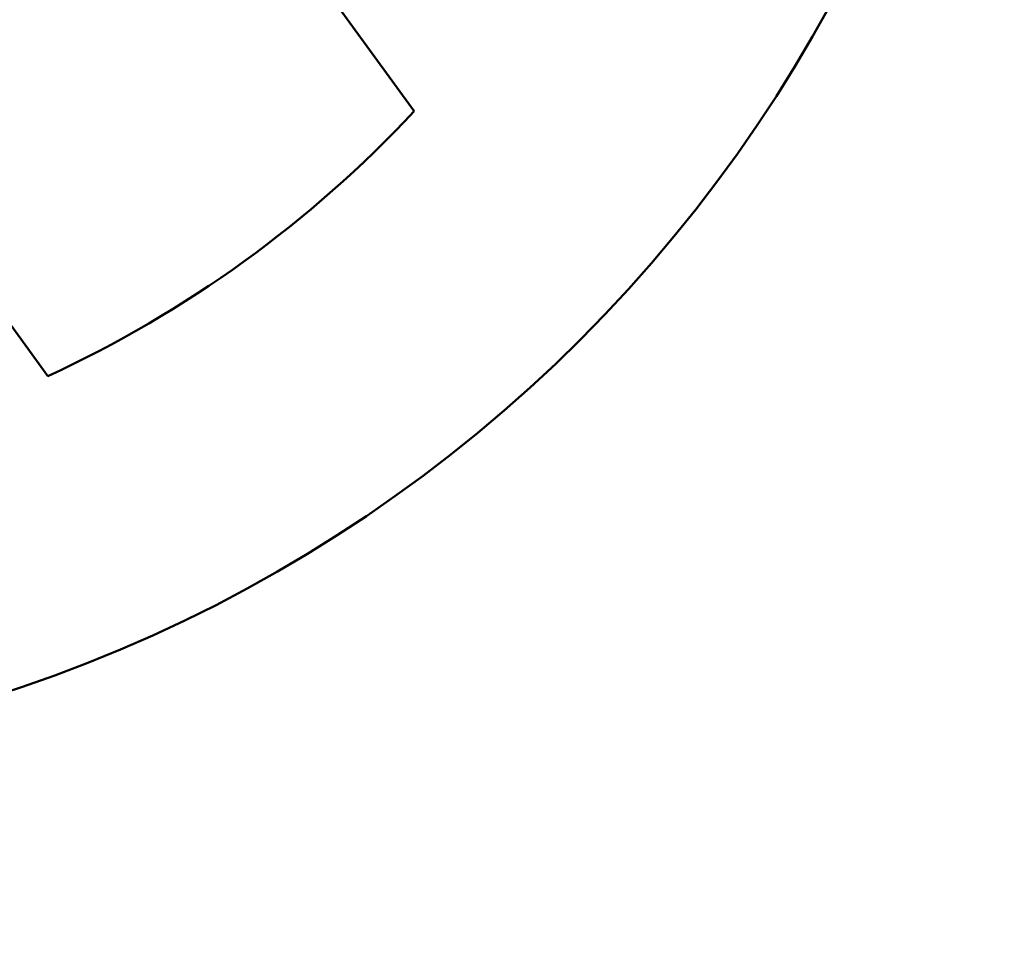
# Model space of a CAD drawing. Units: millimetres. Extents: x -50 to 109, y -46 to 152.
# Tile 5 of 18: x 9 to 31, y -43 to -22. Entities that reach past the tile are written whole.
import ezdxf

# ---------------------------------------------------------------- set-up
doc = ezdxf.new("R2010")
doc.units = ezdxf.units.MM
doc.header["$MEASUREMENT"] = 0
doc.layers.add('M-DIMS', color=2, linetype='Continuous', lineweight=25)
doc.layers.add('M-OUTL', color=7, linetype='Continuous', lineweight=50)
doc.styles.get("Standard").update_dxf_attribs({"font": 'arial.ttf'})
doc.dimstyles.get("Standard").update_dxf_attribs({"dimtxt": 0.18, "dimasz": 0.18, "dimexe": 0.18, "dimexo": 0.0625, "dimgap": 0.09, "dimtad": 0, "dimtih": 1, "dimtoh": 1, "dimdec": 4, "dimzin": 0, "dimdsep": 46, "dimtxsty": 'Standard', "dimcen": 0.09, "dimadec": 0, "dimazin": 0, "dimtfac": 1, "dimtdec": 4, "dimtofl": 0, "dimtmove": 0, "dimatfit": 3, "dimfxl": 1, "dimtolj": 1, "dimtzin": 0, "dimarcsym": 0})

# ---------------------------------------------------------------- blocks, each defined once
blk = doc.blocks.new('*U1')
for p, q in [((-5, 2.851), (-5, -3.294)), ((5, 2.824), (5, -3.323))]:
    blk.add_line(p, q)
blk.add_arc((-0.069, -22.677), 26, 78.7582, 100.9333)
blk = doc.blocks.new('*U2')
at = {"layer": 'M-OUTL', "color": 0, "linetype": 'ByBlock', "lineweight": -2, "transparency": 16777216, "rotation": 216}
blk.add_blockref('*U1', (12.307, -25), dxfattribs=at)
blk = doc.blocks.new('*D23')
at = {"layer": 'Defpoints', "color": 0, "transparency": 16777216}
for p in [(24.75, 12.317), (-26.598, -25.885)]:
    blk.add_point(p, dxfattribs=at)
at = {"layer": 'M-DIMS', "color": 0, "lineweight": -2, "transparency": 16777216}
for p, q in [((-0.924, -6.874), (-0.924, -6.694)), ((-1.014, -6.784), (-0.834, -6.784)), ((-30.604, -28.865), (-26.742, -25.992)), ((-30.784, -28.865), (-30.604, -28.865))]:
    blk.add_line(p, q, dxfattribs=at)
at = {"layer": 'M-DIMS', "color": 0, "transparency": 16777216}
blk.add_solid([(-26.76, -25.968), (-26.724, -26.016), (-26.598, -25.885)], dxfattribs=at)
at = {"layer": 'M-DIMS', "color": 0, "transparency": 16777216, "insert": (-34.648, -28.865), "char_height": 0.18, "attachment_point": 5}
blk.add_mtext('\\A1;{\\H16.66667x;%%C64}', dxfattribs=at)
blk = doc.blocks.new('*D29')
at = {"layer": 'Defpoints', "color": 0, "transparency": 16777216}
for p in [(21.684, 15.863), (-23.531, -29.431)]:
    blk.add_point(p, dxfattribs=at)
at = {"layer": 'M-DIMS', "color": 0, "lineweight": -2, "transparency": 16777216}
for p, q in [((-0.924, -6.874), (-0.924, -6.694)), ((-1.014, -6.784), (-0.834, -6.784)), ((-37.096, -43.02), (-23.658, -29.559)), ((-37.276, -43.02), (-37.096, -43.02))]:
    blk.add_line(p, q, dxfattribs=at)
at = {"layer": 'M-DIMS', "color": 0, "transparency": 16777216}
blk.add_solid([(-23.68, -29.537), (-23.637, -29.58), (-23.531, -29.431)], dxfattribs=at)
at = {"layer": 'M-DIMS', "color": 0, "transparency": 16777216, "insert": (-37.592, -43.02), "char_height": 0.18, "attachment_point": 5}
blk.add_mtext('\\A1;∅64', dxfattribs=at)

msp = doc.modelspace()

# ---------------------------------------------------------------- linework, layer by layer
at = {"layer": 'M-OUTL'}
msp.add_circle((-0.92366, -6.78396), 32, dxfattribs=at)

# ---------------------------------------------------------------- block references
msp.add_blockref('*U2', (0, 0), dxfattribs=at)

# ---------------------------------------------------------------- dimensions: what is measured, and where the dimension line sits
at = {"layer": 'M-DIMS'}
dim = msp.add_diameter_dim_2p(p1=(21.68387, 15.86332), p2=(-23.53119, -29.43125), dimstyle='Standard', override={"dimdec": 0, "dimlfac": 1, "dimrnd": 0, "dimzin": 0, "dimdsep": 46, "dimlunit": 2}, dxfattribs=at)
dim.commit()
dim.dimension.update_dxf_attribs({"geometry": '*D29', "text_midpoint": (-37.59218, -43.01962), "dimtype": 163})
dim = msp.add_diameter_dim_2p(p1=(24.75033, 12.31698), p2=(-26.59765, -25.88491), text='{\\H16.66667x;%%C64}', dimstyle='Standard', override={"dimclrd": 0, "dimclre": 0, "dimclrt": 0}, dxfattribs=at)
dim.commit()
dim.dimension.update_dxf_attribs({"geometry": '*D23', "text_midpoint": (-34.64806, -28.86518), "dimtype": 163})

doc.saveas('drawing.dxf')
